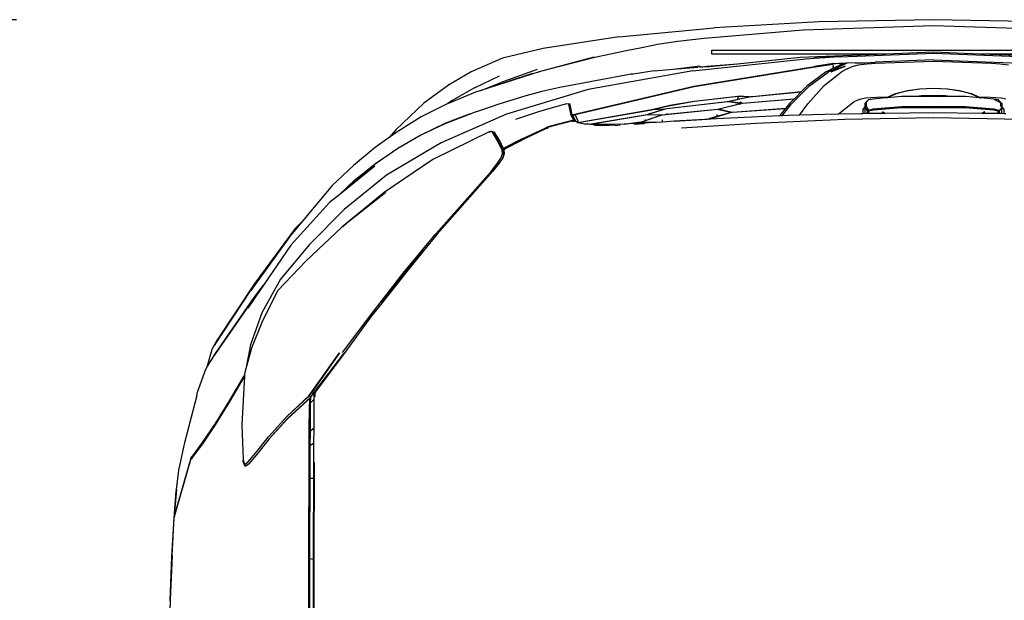
# Model space of a CAD drawing. Units: inches. Extents: x 0 to 4258, y 0 to 3769.
# Tile 13 of 30: x 3726 to 3763, y 3104 to 3126. Entities that reach past the tile are written whole.
import ezdxf

# ---------------------------------------------------------------- set-up
doc = ezdxf.new("R2010")
doc.units = ezdxf.units.IN
doc.header["$MEASUREMENT"] = 0
doc.layers.get('0').update_dxf_attribs({"color": 16})
doc.layers.add('A-ANNO-DIMS', color=250, linetype='Continuous', lineweight=18)
doc.layers.add('C-PKNG-VEHI', color=8, linetype='Continuous', lineweight=18)
doc.layers.add('Edges', color=250, linetype='Continuous')
doc.styles.get("Standard").update_dxf_attribs({"font": 'arial.ttf'})
doc.dimstyles.get("Standard").update_dxf_attribs({"dimtxt": 7, "dimasz": 0.18, "dimexe": 0.18, "dimexo": 0.0625, "dimgap": 0.09, "dimtad": 0, "dimtih": 1, "dimtoh": 1, "dimzin": 0, "dimdsep": 46, "dimlunit": 3, "dimtxsty": 'Standard', "dimcen": 0.09, "dimadec": 0, "dimazin": 0, "dimtfac": 1, "dimtofl": 0, "dimtmove": 0, "dimatfit": 3, "dimfxl": 1, "dimtolj": 1, "dimtzin": 0, "dimarcsym": 0})

# ---------------------------------------------------------------- blocks, each defined once
blk = doc.blocks.new('Nissan Qashqai pl')
at = {"layer": 'Edges'}
for p, q in [((7.3216, 11.6621), (7.3216, 12.1821)), ((7.3261, 12.1821), (7.3261, 11.9779)), ((7.3302, 12.0785), (7.3261, 11.9779)), ((7.298, 12.075), (7.2928, 11.9221)), ((7.2884, 12.0562), (7.2857, 11.9221)), ((7.3251, 11.9221), (7.3291, 12.0316)), ((7.3329, 11.9221), (7.3365, 12.0237)), ((7.4002, 11.9221), (7.4025, 12.026)), ((7.3373, 12.0004), (7.3386, 12.01)), ((7.3367, 11.99), (7.3373, 12.0004)), ((7.3768, 11.9954), (7.3775, 12.0015)), ((7.3775, 12.0015), (7.3786, 12.007)), ((7.3798, 11.9983), (7.3787, 11.9928)), ((7.3808, 11.9993), (7.3798, 11.9983)), ((7.3807, 11.9991), (7.3798, 11.9983)), ((7.38, 11.9953), (7.383, 12.0011)), ((7.3807, 11.9991), (7.3808, 11.9993)), ((7.381, 11.9993), (7.3807, 11.9991)), ((7.3808, 11.9993), (7.384, 12.0021)), ((7.381, 11.9993), (7.3808, 11.9993)), ((7.383, 12.0011), (7.381, 11.9993)), ((7.3866, 12.0011), (7.383, 12.0011)), ((7.384, 12.0021), (7.387, 12.0021)), ((7.3868, 12.002), (7.3866, 12.0011)), ((7.3875, 12.0011), (7.3866, 12.0011)), ((7.387, 12.0021), (7.3868, 12.002)), ((7.3909, 12.0051), (7.387, 12.0021)), ((7.387, 12.0021), (7.3885, 12.0021)), ((7.3885, 12.0021), (7.3925, 11.9993)), ((7.3955, 12.0021), (7.3885, 12.0021)), ((7.3904, 11.9928), (7.3916, 11.9983)), ((7.3956, 12.0051), (7.3909, 12.0051)), ((7.3929, 11.9981), (7.3917, 11.9926)), ((7.3925, 11.9993), (7.3958, 11.9993)), ((7.3925, 11.9993), (7.3929, 11.9981)), ((7.3958, 11.9981), (7.3929, 11.9981)), ((7.3955, 12.0021), (7.3958, 12.0018)), ((7.3959, 12.0049), (7.3956, 12.0051)), ((7.3959, 12.0051), (7.3956, 12.0051)), ((7.3958, 11.9981), (7.3956, 11.9801)), ((7.3959, 12.0049), (7.3958, 12.0018)), ((7.3958, 12.0018), (7.3958, 11.9993)), ((7.3958, 11.9993), (7.3958, 11.9981)), ((7.3959, 12.0071), (7.3959, 12.0051)), ((7.3959, 12.0051), (7.3959, 12.0049)), ((7.3343, 11.9221), (7.3367, 11.99)), ((7.3761, 11.9751), (7.3765, 11.989)), ((7.3765, 11.989), (7.3768, 11.9954)), ((7.3787, 11.9928), (7.3774, 11.9778)), ((7.3787, 11.9928), (7.38, 11.9953)), ((7.3876, 11.9595), (7.3904, 11.9928)), ((7.3917, 11.9926), (7.3889, 11.9594)), ((7.3261, 11.9764), (7.3238, 11.9221)), ((7.3261, 11.9764), (7.3261, 11.9779)), ((7.3724, 11.9667), (7.3761, 11.9751)), ((7.3771, 11.9757), (7.3727, 11.9658)), ((7.3773, 11.9759), (7.3759, 11.9595)), ((7.3761, 11.9751), (7.3769, 11.9767)), ((7.3769, 11.9767), (7.3771, 11.977)), ((7.3774, 11.9778), (7.3771, 11.9771)), ((7.3771, 11.9771), (7.3774, 11.9774)), ((7.3771, 11.9771), (7.3771, 11.977)), ((7.3773, 11.9759), (7.3771, 11.9757)), ((7.3774, 11.9774), (7.3773, 11.9759)), ((7.3774, 11.9774), (7.3774, 11.9778)), ((7.3938, 11.9823), (7.3956, 11.9801)), ((7.3956, 11.9788), (7.3938, 11.981)), ((7.3956, 11.9788), (7.3951, 11.9221)), ((7.3956, 11.9801), (7.3956, 11.9788)), ((7.369, 11.9536), (7.3724, 11.9667)), ((7.3727, 11.9658), (7.3693, 11.953)), ((7.3668, 11.9384), (7.369, 11.9536)), ((7.3693, 11.953), (7.3672, 11.9381)), ((7.3759, 11.9595), (7.3759, 11.9417)), ((7.3876, 11.8847), (7.3876, 11.9595)), ((7.3889, 11.9594), (7.3889, 11.8848)), ((7.3759, 11.9417), (7.3751, 11.9363)), ((7.3759, 11.9417), (7.3759, 11.9303)), ((7.3661, 11.9221), (7.3668, 11.9384)), ((7.3672, 11.9381), (7.3665, 11.9221)), ((7.3751, 11.9363), (7.3745, 11.9221)), ((7.3755, 11.9221), (7.3759, 11.9303)), ((7.3759, 11.9303), (7.3759, 11.9139)), ((7.2857, 11.9221), (7.2884, 11.7879)), ((7.2928, 11.9221), (7.298, 11.7692)), ((7.3238, 11.9221), (7.3261, 11.8662)), ((7.3291, 11.8126), (7.3251, 11.9221)), ((7.3329, 11.9221), (7.3354, 11.8539)), ((7.3367, 11.8541), (7.3343, 11.9221)), ((7.3668, 11.9057), (7.3661, 11.9221)), ((7.3665, 11.9221), (7.3672, 11.9061)), ((7.3745, 11.9221), (7.3751, 11.9078)), ((7.3759, 11.9139), (7.3755, 11.9221)), ((7.3951, 11.9221), (7.3956, 11.8653)), ((7.4025, 11.8181), (7.4002, 11.9221)), ((7.369, 11.8905), (7.3668, 11.9057)), ((7.3672, 11.9061), (7.3693, 11.8911)), ((7.3751, 11.9078), (7.3759, 11.9025)), ((7.3759, 11.9139), (7.3759, 11.9025)), ((7.3759, 11.9025), (7.3759, 11.8847)), ((7.3724, 11.8775), (7.369, 11.8905)), ((7.3693, 11.8911), (7.3727, 11.8783)), ((7.3759, 11.8847), (7.3773, 11.8682)), ((7.3904, 11.8513), (7.3876, 11.8847)), ((7.3889, 11.8848), (7.3917, 11.8516)), ((7.3761, 11.8691), (7.3724, 11.8775)), ((7.3727, 11.8783), (7.3771, 11.8685)), ((7.3261, 11.8662), (7.3302, 11.7656)), ((7.3261, 11.8662), (7.3261, 11.6621)), ((7.3765, 11.8551), (7.3761, 11.8691)), ((7.3769, 11.8674), (7.3761, 11.8691)), ((7.3771, 11.8671), (7.3769, 11.8674)), ((7.3771, 11.8685), (7.3773, 11.8682)), ((7.3771, 11.8671), (7.3771, 11.8671)), ((7.3771, 11.8671), (7.3774, 11.8664)), ((7.3774, 11.8668), (7.3771, 11.8671)), ((7.3773, 11.8682), (7.3774, 11.8668)), ((7.3774, 11.8668), (7.3774, 11.8664)), ((7.3774, 11.8664), (7.3787, 11.8513)), ((7.3938, 11.8632), (7.3956, 11.8653)), ((7.3956, 11.864), (7.3938, 11.8619)), ((7.3956, 11.8653), (7.3956, 11.864)), ((7.3956, 11.864), (7.3958, 11.8461)), ((7.3361, 11.8416), (7.3354, 11.8539)), ((7.3373, 11.8438), (7.3367, 11.8541)), ((7.3768, 11.8488), (7.3765, 11.8551)), ((7.3775, 11.8427), (7.3768, 11.8488)), ((7.3787, 11.8513), (7.3798, 11.8459)), ((7.3916, 11.8459), (7.3904, 11.8513)), ((7.3917, 11.8516), (7.3929, 11.8461)), ((7.3362, 11.8301), (7.3361, 11.8416)), ((7.3386, 11.8342), (7.3373, 11.8438)), ((7.3786, 11.8372), (7.3775, 11.8427)), ((7.3801, 11.8327), (7.3786, 11.8372)), ((7.3798, 11.8459), (7.3808, 11.8448)), ((7.3808, 11.8448), (7.3807, 11.8451)), ((7.3808, 11.8448), (7.381, 11.8448)), ((7.384, 11.8421), (7.3808, 11.8448)), ((7.383, 11.8431), (7.3875, 11.8431)), ((7.387, 11.8421), (7.384, 11.8421)), ((7.387, 11.8421), (7.3909, 11.8391)), ((7.3885, 11.8421), (7.387, 11.8421)), ((7.3875, 11.8431), (7.3916, 11.8459)), ((7.3925, 11.8448), (7.3885, 11.8421)), ((7.3955, 11.8421), (7.3885, 11.8421)), ((7.3909, 11.8391), (7.3956, 11.8391)), ((7.3929, 11.8461), (7.3925, 11.8448)), ((7.3958, 11.8448), (7.3925, 11.8448)), ((7.3929, 11.8461), (7.3958, 11.8461)), ((7.3958, 11.8423), (7.3955, 11.8421)), ((7.3956, 11.8391), (7.3959, 11.8392)), ((7.3956, 11.8391), (7.3959, 11.8391)), ((7.3958, 11.8461), (7.3958, 11.8448)), ((7.3958, 11.8448), (7.3958, 11.8423)), ((7.3958, 11.8423), (7.3959, 11.8392)), ((7.3959, 11.8392), (7.3959, 11.8391)), ((7.3959, 11.8391), (7.3959, 11.8371)), ((7.3959, 11.8371), (7.3966, 11.8103)), ((7.3362, 11.8301), (7.3365, 11.8204)), ((7.3407, 11.8266), (7.3386, 11.8342)), ((7.3432, 11.821), (7.3407, 11.8266)), ((7.3818, 11.8291), (7.3801, 11.8327)), ((7.3966, 11.8103), (7.3818, 11.8291)), ((7.3291, 11.8126), (7.3294, 11.8057)), ((7.3362, 11.8194), (7.3365, 11.8204)), ((7.3367, 11.8196), (7.3362, 11.8194)), ((7.3365, 11.812), (7.3362, 11.8194)), ((7.3365, 11.8204), (7.3471, 11.7987)), ((7.3369, 11.8155), (7.3374, 11.8165)), ((7.3369, 11.8113), (7.3369, 11.8155)), ((7.3369, 11.8155), (7.338, 11.8151)), ((7.3374, 11.8165), (7.338, 11.8151)), ((7.338, 11.8151), (7.343, 11.8045)), ((7.3401, 11.8186), (7.3431, 11.8112)), ((7.347, 11.8021), (7.3401, 11.8186)), ((7.3432, 11.821), (7.3468, 11.8142)), ((7.363, 11.794), (7.3468, 11.8142)), ((7.4072, 11.7142), (7.4025, 11.8181)), ((7.3301, 11.7949), (7.3294, 11.8057)), ((7.3295, 11.8012), (7.3309, 11.7822)), ((7.3295, 11.8012), (7.3301, 11.7949)), ((7.3369, 11.8047), (7.3365, 11.812)), ((7.3369, 11.8113), (7.3377, 11.8044)), ((7.3369, 11.8047), (7.3405, 11.7825)), ((7.3377, 11.8042), (7.3377, 11.8044)), ((7.341, 11.7837), (7.3377, 11.8042)), ((7.343, 11.8045), (7.3396, 11.8043)), ((7.3396, 11.8043), (7.3431, 11.8042)), ((7.343, 11.8045), (7.3431, 11.8042)), ((7.3431, 11.8112), (7.347, 11.8021)), ((7.3431, 11.8042), (7.3469, 11.7961)), ((7.3966, 11.8103), (7.3978, 11.7651)), ((7.3309, 11.7822), (7.3301, 11.7949)), ((7.3469, 11.7961), (7.3631, 11.774)), ((7.3633, 11.7767), (7.3471, 11.7987)), ((7.3842, 11.7749), (7.363, 11.794)), ((7.2884, 11.7879), (7.2951, 11.6651)), ((7.3317, 11.7724), (7.3309, 11.7822)), ((7.3635, 11.6409), (7.3405, 11.7825)), ((7.3426, 11.7735), (7.341, 11.7837)), ((7.298, 11.7692), (7.3078, 11.6532)), ((7.3455, 11.64), (7.3317, 11.7724)), ((7.364, 11.6413), (7.3426, 11.7735)), ((7.3631, 11.774), (7.3701, 11.7671)), ((7.3845, 11.7558), (7.3633, 11.7767)), ((7.3759, 11.7101), (7.3701, 11.7671)), ((7.3701, 11.7671), (7.3704, 11.7668)), ((7.3704, 11.7668), (7.3761, 11.71)), ((7.3704, 11.7668), (7.3783, 11.759)), ((7.3978, 11.7651), (7.3842, 11.7749)), ((7.3302, 11.7656), (7.3378, 11.6921)), ((7.3836, 11.6983), (7.3783, 11.759)), ((7.3783, 11.759), (7.3788, 11.7585)), ((7.3788, 11.7585), (7.384, 11.6982)), ((7.3788, 11.7585), (7.3841, 11.7532)), ((7.3985, 11.7448), (7.3845, 11.7558)), ((7.3978, 11.7651), (7.3982, 11.7521)), ((7.3841, 11.7532), (7.3896, 11.7488)), ((7.3941, 11.6865), (7.3896, 11.7488)), ((7.3896, 11.7488), (7.3903, 11.7483)), ((7.3903, 11.7483), (7.3945, 11.6865)), ((7.3903, 11.7483), (7.3986, 11.7417)), ((7.3982, 11.7521), (7.3985, 11.7448)), ((7.3985, 11.7448), (7.3986, 11.7417)), ((7.3986, 11.7417), (7.4018, 11.6678)), ((7.376, 11.7081), (7.3759, 11.7101)), ((7.3761, 11.71), (7.3763, 11.7081)), ((7.4124, 11.6265), (7.4072, 11.7142)), ((7.375, 11.6957), (7.376, 11.7081)), ((7.3762, 11.7062), (7.3757, 11.6959)), ((7.3762, 11.7062), (7.3764, 11.7061)), ((7.3763, 11.7081), (7.3813, 11.6842)), ((7.3764, 11.7061), (7.3792, 11.6924)), ((7.3824, 11.6955), (7.3836, 11.6983)), ((7.3835, 11.6973), (7.3824, 11.6955)), ((7.3835, 11.6973), (7.3836, 11.6983)), ((7.3836, 11.6975), (7.3835, 11.6973)), ((7.3836, 11.6975), (7.3836, 11.6983)), ((7.384, 11.6982), (7.3836, 11.6975)), ((7.3378, 11.6921), (7.3407, 11.6563)), ((7.3378, 11.6921), (7.34, 11.671)), ((7.3813, 11.642), (7.375, 11.6957)), ((7.3757, 11.6959), (7.3756, 11.6933)), ((7.3792, 11.6924), (7.3756, 11.6933)), ((7.3756, 11.6933), (7.3815, 11.6413)), ((7.3757, 11.6959), (7.3757, 11.6959)), ((7.3812, 11.6823), (7.3792, 11.6924)), ((7.3817, 11.6844), (7.3832, 11.6949)), ((7.3838, 11.6944), (7.382, 11.6823)), ((7.3834, 11.6959), (7.3824, 11.6955)), ((7.3824, 11.6955), (7.3832, 11.6949)), ((7.3832, 11.695), (7.3824, 11.6955)), ((7.3832, 11.695), (7.3834, 11.6959)), ((7.3838, 11.6947), (7.3832, 11.695)), ((7.3832, 11.6949), (7.3838, 11.6944)), ((7.3837, 11.696), (7.3834, 11.6959)), ((7.3844, 11.6963), (7.3837, 11.696)), ((7.3838, 11.6947), (7.3837, 11.696)), ((7.3843, 11.6944), (7.3838, 11.6947)), ((7.3843, 11.6942), (7.3838, 11.6944)), ((7.3843, 11.6944), (7.3844, 11.6963)), ((7.3843, 11.6942), (7.3843, 11.6944)), ((7.3877, 11.6803), (7.3843, 11.6942)), ((7.3844, 11.6963), (7.3903, 11.6725)), ((7.3939, 11.6846), (7.3941, 11.6865)), ((7.3945, 11.6865), (7.3951, 11.6835)), ((7.3815, 11.6804), (7.3812, 11.6823)), ((7.3813, 11.6842), (7.3817, 11.6844)), ((7.3817, 11.6841), (7.3813, 11.6842)), ((7.3899, 11.6094), (7.3815, 11.6804)), ((7.3817, 11.6841), (7.3817, 11.6844)), ((7.382, 11.6823), (7.382, 11.6803)), ((7.382, 11.6803), (7.3903, 11.6095)), ((7.3874, 11.6803), (7.3877, 11.6803)), ((7.3901, 11.6707), (7.3877, 11.6803)), ((7.3909, 11.6728), (7.3939, 11.6846)), ((7.3943, 11.6827), (7.3913, 11.6705)), ((7.3943, 11.6827), (7.3949, 11.6826)), ((7.3943, 11.6827), (7.395, 11.6825)), ((7.395, 11.6825), (7.3949, 11.6826)), ((7.399, 11.6686), (7.395, 11.6825)), ((7.3951, 11.6835), (7.4021, 11.6609)), ((7.3059, 11.5532), (7.2951, 11.6651)), ((7.3261, 11.6621), (7.3216, 11.6621)), ((7.34, 11.671), (7.341, 11.6594)), ((7.3905, 11.6687), (7.3901, 11.6707)), ((7.3909, 11.6728), (7.3903, 11.6725)), ((7.3909, 11.6725), (7.3903, 11.6725)), ((7.3966, 11.6095), (7.3905, 11.6687)), ((7.3909, 11.6725), (7.3909, 11.6728)), ((7.3913, 11.6705), (7.3911, 11.6687)), ((7.3911, 11.6687), (7.3977, 11.6042)), ((7.399, 11.6686), (7.3967, 11.6686)), ((7.4017, 11.6592), (7.399, 11.6686)), ((7.4018, 11.6678), (7.4022, 11.6609)), ((7.3078, 11.6532), (7.3113, 11.6224)), ((7.3407, 11.6563), (7.3413, 11.6509)), ((7.341, 11.6594), (7.3413, 11.6511)), ((7.341, 11.648), (7.3413, 11.6509)), ((7.3413, 11.6511), (7.3413, 11.6509)), ((7.3413, 11.6509), (7.3415, 11.6488)), ((7.4022, 11.6571), (7.4017, 11.6592)), ((7.4022, 11.6609), (7.4021, 11.6609)), ((7.4022, 11.6609), (7.4021, 11.6609)), ((7.4022, 11.6609), (7.4048, 11.618)), ((7.4022, 11.6609), (7.4022, 11.6609)), ((7.4048, 11.618), (7.4022, 11.6571)), ((7.3401, 11.648), (7.34, 11.648)), ((7.3438, 11.6167), (7.34, 11.648)), ((7.341, 11.648), (7.3401, 11.648)), ((7.3414, 11.648), (7.341, 11.648)), ((7.341, 11.648), (7.3414, 11.648)), ((7.3438, 11.6167), (7.3412, 11.646)), ((7.3455, 11.64), (7.3676, 11.5172)), ((7.3971, 11.4981), (7.3635, 11.6409)), ((7.3968, 11.5018), (7.364, 11.6413)), ((7.3869, 11.6094), (7.3813, 11.642)), ((7.3815, 11.6413), (7.3864, 11.6131)), ((7.3113, 11.6224), (7.3149, 11.5984)), ((7.3457, 11.5947), (7.3438, 11.6167)), ((7.4048, 11.618), (7.4057, 11.6042)), ((7.3864, 11.6131), (7.3909, 11.5933)), ((7.3912, 11.5914), (7.3869, 11.6094)), ((7.3901, 11.6073), (7.3899, 11.6094)), ((7.391, 11.5935), (7.3901, 11.6073)), ((7.3903, 11.6095), (7.3908, 11.6076)), ((7.3906, 11.6055), (7.391, 11.6055)), ((7.3906, 11.6055), (7.391, 11.6054)), ((7.3906, 11.6055), (7.3914, 11.5914)), ((7.3908, 11.6076), (7.3965, 11.5881)), ((7.391, 11.6054), (7.391, 11.6055)), ((7.3967, 11.5862), (7.391, 11.6054)), ((7.3966, 11.6095), (7.3957, 11.6095)), ((7.3972, 11.6042), (7.3966, 11.6095)), ((7.3149, 11.5984), (7.3186, 11.58)), ((7.3457, 11.5947), (7.3494, 11.57)), ((7.391, 11.5935), (7.3909, 11.5933)), ((7.391, 11.5934), (7.3909, 11.5933)), ((7.3968, 11.5882), (7.3972, 11.6021)), ((7.3972, 11.6021), (7.3972, 11.6042)), ((7.3977, 11.6003), (7.3973, 11.5862)), ((7.3977, 11.6042), (7.3982, 11.6022)), ((7.3977, 11.6003), (7.3983, 11.6002)), ((7.3977, 11.6003), (7.3983, 11.6001)), ((7.3982, 11.6022), (7.4048, 11.5829)), ((7.3983, 11.6001), (7.3983, 11.6002)), ((7.4038, 11.5843), (7.3983, 11.6001)), ((7.4057, 11.6042), (7.4032, 11.6042)), ((7.4053, 11.5831), (7.4061, 11.5969)), ((7.4057, 11.6042), (7.4061, 11.597)), ((7.4061, 11.5969), (7.4061, 11.597)), ((7.4061, 11.5969), (7.4064, 11.5919)), ((7.3916, 11.5894), (7.3912, 11.5914)), ((7.3914, 11.5914), (7.3917, 11.5895)), ((7.4062, 11.5053), (7.3916, 11.5894)), ((7.3917, 11.5895), (7.4065, 11.505)), ((7.3968, 11.5882), (7.3965, 11.5881)), ((7.3971, 11.5842), (7.3967, 11.5862)), ((7.3968, 11.5882), (7.3973, 11.5884)), ((7.4083, 11.5184), (7.3971, 11.5842)), ((7.3973, 11.5862), (7.3975, 11.5843)), ((7.3975, 11.5843), (7.4084, 11.5198)), ((7.4038, 11.5843), (7.4028, 11.5843)), ((7.4049, 11.5811), (7.4038, 11.5843)), ((7.4053, 11.5831), (7.4048, 11.5829)), ((7.4053, 11.583), (7.4048, 11.5829)), ((7.406, 11.5834), (7.4053, 11.5831)), ((7.406, 11.5833), (7.4053, 11.583)), ((7.4053, 11.583), (7.4053, 11.5831)), ((7.406, 11.5833), (7.4058, 11.581)), ((7.4064, 11.5919), (7.406, 11.5834)), ((7.406, 11.5834), (7.406, 11.5833)), ((7.4064, 11.5919), (7.4069, 11.5844)), ((7.4069, 11.5844), (7.4079, 11.5644)), ((7.4081, 11.5711), (7.4075, 11.5828)), ((7.3186, 11.58), (7.3223, 11.5616)), ((7.3494, 11.57), (7.3497, 11.5674)), ((7.3494, 11.57), (7.3498, 11.5674)), ((7.4054, 11.5791), (7.4049, 11.5811)), ((7.4081, 11.5593), (7.4054, 11.5791)), ((7.4058, 11.581), (7.4059, 11.579)), ((7.4059, 11.579), (7.4079, 11.5644)), ((7.3223, 11.5616), (7.3261, 11.5433)), ((7.3497, 11.5674), (7.3653, 11.4838)), ((7.4079, 11.5644), (7.4081, 11.5604)), ((7.4079, 11.5644), (7.4081, 11.5629)), ((7.4081, 11.5604), (7.4081, 11.5593)), ((7.4081, 11.5593), (7.4087, 11.5405)), ((7.3059, 11.5532), (7.3193, 11.4645)), ((7.4092, 11.5416), (7.409, 11.5485)), ((7.4096, 11.549), (7.4092, 11.5521)), ((7.4093, 11.5546), (7.4095, 11.5529)), ((7.3261, 11.5433), (7.33, 11.5249)), ((7.4087, 11.5405), (7.4087, 11.5246)), ((7.4092, 11.5258), (7.4092, 11.5416)), ((7.3297, 11.5237), (7.3467, 11.4596)), ((7.33, 11.5249), (7.3467, 11.4596)), ((7.4087, 11.5246), (7.4084, 11.5198)), ((7.4091, 11.5235), (7.4092, 11.5258)), ((7.3676, 11.5172), (7.3963, 11.4215)), ((7.408, 11.5129), (7.4066, 11.5052)), ((7.4083, 11.5184), (7.408, 11.5129)), ((7.4084, 11.5198), (7.4083, 11.5184)), ((7.4046, 11.5053), (7.3968, 11.5018)), ((7.398, 11.4993), (7.3968, 11.5018)), ((7.398, 11.4993), (7.4048, 11.5024)), ((7.4012, 11.5001), (7.4033, 11.5014)), ((7.403, 11.5005), (7.4026, 11.5002)), ((7.403, 11.5005), (7.4028, 11.5004)), ((7.4033, 11.5007), (7.403, 11.5005)), ((7.4033, 11.5014), (7.4042, 11.502)), ((7.4042, 11.502), (7.4033, 11.5007)), ((7.4033, 11.5005), (7.4033, 11.5007)), ((7.4034, 11.5005), (7.4033, 11.5005)), ((7.4101, 11.4733), (7.4033, 11.5005)), ((7.4043, 11.5016), (7.404, 11.5012)), ((7.4043, 11.5014), (7.404, 11.5012)), ((7.404, 11.5012), (7.4108, 11.4738)), ((7.4042, 11.502), (7.4044, 11.502)), ((7.4043, 11.5016), (7.4042, 11.502)), ((7.4044, 11.502), (7.4043, 11.5016)), ((7.4046, 11.5016), (7.4043, 11.5014)), ((7.4043, 11.5014), (7.4043, 11.5016)), ((7.4045, 11.5008), (7.4043, 11.5014)), ((7.4046, 11.5023), (7.4044, 11.502)), ((7.4044, 11.502), (7.4046, 11.502)), ((7.4048, 11.5008), (7.4045, 11.5008)), ((7.405, 11.4985), (7.4045, 11.5008)), ((7.4062, 11.5053), (7.4046, 11.5053)), ((7.4046, 11.5023), (7.4048, 11.5024)), ((7.405, 11.5023), (7.4046, 11.5023)), ((7.4046, 11.5023), (7.4046, 11.502)), ((7.4046, 11.502), (7.4047, 11.5018)), ((7.4046, 11.502), (7.4048, 11.502)), ((7.4047, 11.5018), (7.4046, 11.5016)), ((7.4048, 11.502), (7.4047, 11.5018)), ((7.4048, 11.5024), (7.4052, 11.5027)), ((7.4052, 11.5026), (7.4048, 11.5024)), ((7.405, 11.5023), (7.4048, 11.502)), ((7.4052, 11.5026), (7.405, 11.5023)), ((7.4063, 11.5047), (7.4052, 11.5027)), ((7.4052, 11.5027), (7.4052, 11.5026)), ((7.4063, 11.5047), (7.4062, 11.5053)), ((7.4065, 11.505), (7.4063, 11.5047)), ((7.4066, 11.5052), (7.4065, 11.505)), ((7.3853, 11.4958), (7.3841, 11.4956)), ((7.3844, 11.4916), (7.3841, 11.4956)), ((7.3846, 11.4946), (7.3844, 11.4916)), ((7.3844, 11.4916), (7.3914, 11.4667)), ((7.3976, 11.4971), (7.3846, 11.4946)), ((7.3853, 11.4958), (7.3846, 11.4946)), ((7.3853, 11.4958), (7.3971, 11.4981)), ((7.3971, 11.4981), (7.3983, 11.4983)), ((7.4026, 11.5002), (7.3976, 11.4971)), ((7.4012, 11.5001), (7.398, 11.4993)), ((7.3983, 11.4983), (7.4012, 11.5001)), ((7.3653, 11.4838), (7.3699, 11.4629)), ((7.3914, 11.4667), (7.3925, 11.4629)), ((7.4115, 11.4695), (7.4101, 11.4733)), ((7.4108, 11.4738), (7.4122, 11.47)), ((7.4131, 11.4659), (7.4115, 11.4695)), ((7.4122, 11.47), (7.4139, 11.4664)), ((7.4126, 11.47), (7.4125, 11.4702)), ((7.4132, 11.4685), (7.4126, 11.47)), ((7.4255, 11.4398), (7.4131, 11.4659)), ((7.4139, 11.4664), (7.4267, 11.4401)), ((7.3193, 11.4645), (7.3309, 11.4166)), ((7.344, 11.4572), (7.3596, 11.4139)), ((7.3489, 11.4517), (7.3467, 11.4596)), ((7.3467, 11.4596), (7.3686, 11.3913)), ((7.3699, 11.4629), (7.375, 11.4442)), ((7.3925, 11.4629), (7.3937, 11.4591)), ((7.3937, 11.4591), (7.4029, 11.4321)), ((7.3489, 11.4517), (7.3686, 11.3913)), ((7.375, 11.4442), (7.3799, 11.4278)), ((7.4255, 11.4398), (7.4367, 11.4174)), ((7.4379, 11.4179), (7.4267, 11.4401)), ((7.3799, 11.4278), (7.3845, 11.4136)), ((7.3963, 11.4215), (7.4302, 11.3449)), ((7.4375, 11.42), (7.4384, 11.4182)), ((7.3309, 11.4166), (7.347, 11.3798)), ((7.3655, 11.3837), (7.3514, 11.4133)), ((7.3686, 11.3913), (7.3596, 11.4139)), ((7.3845, 11.4136), (7.3925, 11.3899)), ((7.4282, 11.4113), (7.4169, 11.4044)), ((7.417, 11.4065), (7.4283, 11.4135)), ((7.4296, 11.4129), (7.4183, 11.406)), ((7.4387, 11.4162), (7.4282, 11.4113)), ((7.4283, 11.4135), (7.4359, 11.417)), ((7.4296, 11.4129), (7.4383, 11.417)), ((7.4359, 11.417), (7.4367, 11.4174)), ((7.4383, 11.417), (7.4367, 11.4174)), ((7.4379, 11.4179), (7.4384, 11.4182)), ((7.4389, 11.4173), (7.4379, 11.4179)), ((7.4383, 11.417), (7.4379, 11.4179)), ((7.4389, 11.4173), (7.4383, 11.417)), ((7.4384, 11.4182), (7.4387, 11.4183)), ((7.4387, 11.4183), (7.443, 11.4188)), ((7.4431, 11.4166), (7.4387, 11.4162)), ((7.4389, 11.4173), (7.44, 11.4178)), ((7.4442, 11.4183), (7.44, 11.4178)), ((7.443, 11.4188), (7.4477, 11.4172)), ((7.4479, 11.4149), (7.4431, 11.4166)), ((7.4477, 11.4172), (7.4442, 11.4183)), ((7.4477, 11.4172), (7.4541, 11.4128)), ((7.4541, 11.4108), (7.4479, 11.4149)), ((7.4541, 11.4128), (7.4638, 11.4051)), ((7.4635, 11.4034), (7.4541, 11.4108)), ((7.4167, 11.4049), (7.417, 11.4065)), ((7.4172, 11.4047), (7.4167, 11.4049)), ((7.4169, 11.4036), (7.4167, 11.4049)), ((7.4172, 11.4047), (7.4169, 11.4044)), ((7.4169, 11.4044), (7.4169, 11.4036)), ((7.4172, 11.4018), (7.4169, 11.4036)), ((7.4169, 11.4036), (7.4169, 11.403)), ((7.4169, 11.403), (7.4172, 11.4011)), ((7.4183, 11.406), (7.4172, 11.4047)), ((7.4174, 11.4013), (7.4172, 11.4018)), ((7.4172, 11.4011), (7.4498, 11.3349)), ((7.4174, 11.4013), (7.4175, 11.4012)), ((7.5369, 11.3385), (7.4635, 11.4034)), ((7.4638, 11.4051), (7.5371, 11.34)), ((7.3686, 11.3913), (7.3707, 11.3849)), ((7.3925, 11.3899), (7.3938, 11.3859)), ((7.3938, 11.3859), (7.3951, 11.3822)), ((7.347, 11.3798), (7.3624, 11.3535)), ((7.3655, 11.3837), (7.3805, 11.3576)), ((7.3707, 11.3849), (7.3843, 11.3522)), ((7.3951, 11.3822), (7.3965, 11.3787)), ((7.3962, 11.3781), (7.3965, 11.3787)), ((7.4071, 11.3493), (7.3962, 11.3781)), ((7.3965, 11.3787), (7.3969, 11.3777)), ((7.3969, 11.3777), (7.4078, 11.349)), ((7.3624, 11.3535), (7.3837, 11.3245)), ((7.3805, 11.3576), (7.3843, 11.3522)), ((7.3843, 11.3522), (7.3845, 11.3517)), ((7.3845, 11.3517), (7.3997, 11.3215)), ((7.4205, 11.3212), (7.4071, 11.3493)), ((7.4078, 11.349), (7.4211, 11.321)), ((7.4302, 11.3449), (7.4679, 11.2807)), ((7.5371, 11.34), (7.5568, 11.324)), ((7.4498, 11.3349), (7.4884, 11.2778)), ((7.5827, 11.3001), (7.5369, 11.3385)), ((7.3837, 11.3245), (7.4147, 11.2918)), ((7.3997, 11.3215), (7.4166, 11.2939)), ((7.4363, 11.294), (7.4205, 11.3212)), ((7.4211, 11.321), (7.4369, 11.2938)), ((7.584, 11.3013), (7.5568, 11.324)), ((7.5568, 11.324), (7.5829, 11.303)), ((7.4166, 11.2939), (7.4239, 11.2837)), ((7.4542, 11.2677), (7.4363, 11.294)), ((7.4369, 11.2938), (7.4549, 11.2675)), ((7.6296, 11.2639), (7.5827, 11.3001)), ((7.5829, 11.303), (7.618, 11.275)), ((7.618, 11.275), (7.584, 11.3013)), ((7.4147, 11.2918), (7.4239, 11.2837)), ((7.4239, 11.2837), (7.4354, 11.2675)), ((7.4679, 11.2807), (7.5081, 11.2311)), ((7.4882, 11.2797), (7.5243, 11.2341)), ((7.4884, 11.2778), (7.5289, 11.2283)), ((7.618, 11.275), (7.6301, 11.2654)), ((7.4354, 11.2675), (7.4565, 11.2419)), ((7.4744, 11.2427), (7.4542, 11.2677)), ((7.4549, 11.2675), (7.475, 11.2426)), ((7.4574, 11.267), (7.4885, 11.2283)), ((7.676, 11.2289), (7.6296, 11.2639)), ((7.6301, 11.2654), (7.6306, 11.2651)), ((7.6306, 11.2651), (7.6306, 11.265)), ((7.6306, 11.265), (7.6373, 11.2601)), ((7.6373, 11.2601), (7.6769, 11.2312)), ((7.4565, 11.2419), (7.4801, 11.2168)), ((7.4918, 11.2242), (7.4744, 11.2427)), ((7.475, 11.2426), (7.477, 11.2404)), ((7.477, 11.2404), (7.4765, 11.2411)), ((7.477, 11.2405), (7.4775, 11.2399)), ((7.4784, 11.2388), (7.477, 11.2404)), ((7.477, 11.2404), (7.4775, 11.2399)), ((7.4775, 11.2399), (7.4787, 11.2385)), ((7.4775, 11.2399), (7.4787, 11.2387)), ((7.4787, 11.2387), (7.4782, 11.2392)), ((7.4795, 11.2377), (7.4787, 11.2387)), ((7.4787, 11.2387), (7.4885, 11.2283)), ((7.4885, 11.2283), (7.4918, 11.2242)), ((7.4918, 11.2242), (7.5001, 11.2139)), ((7.5081, 11.2311), (7.5492, 11.1902)), ((7.5243, 11.2341), (7.5286, 11.2296)), ((7.5289, 11.2283), (7.5687, 11.1862)), ((7.7261, 11.1898), (7.6762, 11.2256)), ((7.6762, 11.2256), (7.7233, 11.1928)), ((7.6769, 11.2312), (7.7194, 11.1992)), ((7.7232, 11.1955), (7.6771, 11.2307)), ((7.4801, 11.2168), (7.5217, 11.1823)), ((7.5001, 11.2139), (7.5501, 11.1684)), ((7.5492, 11.1902), (7.59, 11.1565)), ((7.7194, 11.1992), (7.7232, 11.1966)), ((7.7232, 11.1966), (7.7279, 11.1965)), ((7.7281, 11.1918), (7.7232, 11.1955)), ((7.7232, 11.1955), (7.7245, 11.1955)), ((7.7267, 11.1902), (7.7233, 11.1928)), ((7.7247, 11.1954), (7.7245, 11.1955)), ((7.7245, 11.1955), (7.7294, 11.1955)), ((7.7261, 11.1898), (7.7507, 11.1638)), ((7.7286, 11.1881), (7.7267, 11.1902)), ((7.7281, 11.1918), (7.7299, 11.1904)), ((7.7349, 11.1917), (7.7281, 11.1918)), ((7.753, 11.1648), (7.7281, 11.1918)), ((7.7294, 11.1955), (7.731, 11.1955)), ((7.7299, 11.1904), (7.7324, 11.1876)), ((7.7299, 11.1904), (7.7364, 11.1904)), ((7.731, 11.1955), (7.7349, 11.1917)), ((7.731, 11.1955), (7.764, 11.1953)), ((7.768, 11.1915), (7.7349, 11.1917)), ((7.7363, 11.1904), (7.7364, 11.1904)), ((7.7694, 11.1901), (7.7364, 11.1904)), ((7.764, 11.1953), (7.7636, 11.1957)), ((7.768, 11.1915), (7.764, 11.1953)), ((7.764, 11.1953), (7.7662, 11.1953)), ((7.7659, 11.1957), (7.7662, 11.1953)), ((7.7662, 11.1953), (7.7668, 11.1946)), ((7.7662, 11.1953), (7.7811, 11.1952)), ((7.7692, 11.1915), (7.768, 11.1915)), ((7.7694, 11.1901), (7.7687, 11.1908)), ((7.7844, 11.1913), (7.7692, 11.1915)), ((7.7707, 11.1901), (7.7694, 11.1901)), ((7.7851, 11.19), (7.7707, 11.1901)), ((7.7811, 11.1952), (7.7809, 11.1958)), ((7.7814, 11.1946), (7.7811, 11.1952)), ((7.7811, 11.1952), (7.7822, 11.1952)), ((7.7822, 11.1952), (7.7819, 11.1958)), ((7.7822, 11.1952), (7.8057, 11.195)), ((7.7844, 11.1913), (7.7822, 11.1952)), ((7.8078, 11.1911), (7.7844, 11.1913)), ((7.7846, 11.1909), (7.7851, 11.19)), ((7.8083, 11.1898), (7.7851, 11.19)), ((7.8048, 11.1959), (7.8233, 11.1958)), ((7.8057, 11.195), (7.8233, 11.195)), ((7.8233, 11.1911), (7.8078, 11.1911)), ((7.904, 11.1894), (7.8083, 11.1898)), ((7.8233, 11.195), (7.8233, 11.1958)), ((7.8233, 11.1958), (7.9014, 11.1955)), ((7.8233, 11.195), (7.902, 11.1947)), ((7.8233, 11.1911), (7.8233, 11.195)), ((7.8233, 11.1899), (7.8233, 11.1911)), ((7.9036, 11.1907), (7.8233, 11.1911)), ((7.9014, 11.1955), (7.9185, 11.1955)), ((7.902, 11.1947), (7.9183, 11.1947)), ((7.9176, 11.1908), (7.9036, 11.1907)), ((8.0276, 11.1896), (7.904, 11.1894)), ((7.9183, 11.1947), (7.9176, 11.1908)), ((8.0275, 11.1909), (7.9176, 11.1908)), ((7.9185, 11.1955), (7.9183, 11.1947)), ((7.9183, 11.1947), (8.0275, 11.1948)), ((7.9185, 11.1955), (8.0273, 11.1957)), ((7.5304, 11.1737), (7.5217, 11.1823)), ((7.5217, 11.1823), (7.5387, 11.1682)), ((7.5687, 11.1862), (7.6032, 11.1533)), ((7.7507, 11.1638), (7.7286, 11.1881)), ((7.7324, 11.1876), (7.7539, 11.1642)), ((7.5304, 11.1737), (7.5946, 11.1262)), ((7.5387, 11.1682), (7.6031, 11.1217)), ((7.5501, 11.1684), (7.5969, 11.1365)), ((7.59, 11.1565), (7.6295, 11.1344)), ((7.7748, 11.1423), (7.7507, 11.1638)), ((7.753, 11.1648), (7.7772, 11.1431)), ((7.7539, 11.1642), (7.7772, 11.1431)), ((7.6032, 11.1533), (7.6386, 11.1353)), ((7.7772, 11.1431), (7.7959, 11.1281)), ((7.6113, 11.1256), (7.5969, 11.1365)), ((7.5969, 11.1365), (7.6021, 11.1329)), ((7.6021, 11.1329), (7.6118, 11.1255)), ((7.6021, 11.1329), (7.6237, 11.1181)), ((7.6295, 11.1344), (7.667, 11.1212)), ((7.6386, 11.1353), (7.6708, 11.1225)), ((7.7938, 11.1271), (7.7748, 11.1423)), ((7.5946, 11.1262), (7.6608, 11.0825)), ((7.6676, 11.0791), (7.6024, 11.1221)), ((7.6759, 11.0809), (7.6113, 11.1256)), ((7.6118, 11.1255), (7.6799, 11.0783)), ((7.667, 11.1212), (7.6949, 11.1158)), ((7.6708, 11.1225), (7.6949, 11.1158)), ((7.8045, 11.1179), (7.7938, 11.1271)), ((7.7959, 11.1281), (7.8062, 11.1192)), ((7.6949, 11.1158), (7.701, 11.1141)), ((7.701, 11.1141), (7.7024, 11.1141)), ((7.7038, 11.1132), (7.7024, 11.1141)), ((7.7024, 11.1141), (7.7034, 11.114)), ((7.7034, 11.114), (7.7056, 11.1128)), ((7.7034, 11.114), (7.7608, 11.1112)), ((7.7325, 11.0966), (7.7038, 11.1132)), ((7.7056, 11.1128), (7.7341, 11.0963)), ((7.7608, 11.1112), (7.8014, 11.1124)), ((7.8014, 11.1124), (7.8022, 11.1126)), ((7.8022, 11.1126), (7.8072, 11.1141)), ((7.8037, 11.1126), (7.8022, 11.1126)), ((7.8096, 11.1148), (7.8037, 11.1126)), ((7.8072, 11.1141), (7.8045, 11.1179)), ((7.8087, 11.1159), (7.8062, 11.1192)), ((7.8062, 11.1192), (7.8066, 11.1188)), ((7.8066, 11.1188), (7.8096, 11.1148)), ((7.8072, 11.1141), (7.8087, 11.1159)), ((7.7591, 11.08), (7.7325, 11.0966)), ((7.7341, 11.0963), (7.7606, 11.0798)), ((7.6712, 11.0767), (7.6608, 11.0825)), ((7.6721, 11.0762), (7.6712, 11.0767)), ((7.6926, 11.0705), (7.6721, 11.0762)), ((7.6793, 11.0784), (7.6759, 11.0809)), ((7.6802, 11.0782), (7.6793, 11.0784)), ((7.6802, 11.0782), (7.6799, 11.0783)), ((7.6809, 11.0777), (7.6802, 11.0782)), ((7.6926, 11.0705), (7.6809, 11.0777)), ((7.7814, 11.065), (7.7591, 11.08)), ((7.7606, 11.0798), (7.7828, 11.0649)), ((7.6953, 11.0688), (7.6926, 11.0705)), ((7.7223, 11.059), (7.6953, 11.0688)), ((7.797, 11.0534), (7.7814, 11.065)), ((7.7828, 11.0649), (7.7984, 11.0533)), ((7.7262, 11.0581), (7.7223, 11.059)), ((7.7262, 11.0581), (7.7819, 11.0438)), ((7.797, 11.0534), (7.797, 11.0534)), ((7.7998, 11.0513), (7.797, 11.0534)), ((7.7984, 11.0533), (7.8007, 11.0516)), ((7.7998, 11.0513), (7.8676, 11.0318)), ((7.8007, 11.0516), (7.8002, 11.0517)), ((7.8007, 11.0516), (7.8012, 11.0513)), ((7.8681, 11.032), (7.8012, 11.0513)), ((7.7819, 11.0438), (7.7848, 11.043)), ((7.7848, 11.043), (7.8087, 11.038)), ((7.8087, 11.038), (7.8106, 11.0377)), ((7.8107, 11.0377), (7.8106, 11.0377)), ((7.8363, 11.0344), (7.8107, 11.0377)), ((7.8381, 11.0342), (7.8363, 11.0344)), ((7.8363, 11.0344), (7.8676, 11.0318)), ((7.87, 11.0315), (7.8381, 11.0342)), ((7.8681, 11.032), (7.8676, 11.0318)), ((7.8681, 11.032), (7.869, 11.0317)), ((7.9137, 11.0292), (7.869, 11.0317)), ((7.9151, 11.029), (7.87, 11.0315)), ((7.9137, 11.0292), (7.9658, 11.027)), ((7.9668, 11.0268), (7.9151, 11.029)), ((7.9658, 11.027), (8.016, 11.0253))]:
    blk.add_line(p, q, dxfattribs=at)
blk = doc.blocks.new('car')
blk.add_blockref('Nissan Qashqai pl', (-9.7433, -11.9151))
blk = doc.blocks.new('*D66')
at = {"layer": 'A-ANNO-DIMS', "color": 0, "lineweight": -2, "transparency": 16777216}
for p, q in [((3725.517, 3125.846), (3703.936, 3125.846)), ((3704.116, 3125.666), (3704.116, 3058.01)), ((3704.116, 2982.935), (3704.116, 3050.591)), ((3725.517, 2982.755), (3703.936, 2982.755))]:
    blk.add_line(p, q, dxfattribs=at)
at = {"layer": 'A-ANNO-DIMS', "color": 0, "transparency": 16777216}
for points in [[(3704.086, 3125.666), (3704.146, 3125.666), (3704.116, 3125.846)], [(3704.086, 2982.935), (3704.146, 2982.935), (3704.116, 2982.755)]]:
    blk.add_solid(points, dxfattribs=at)
at = {"layer": 'Defpoints', "color": 0, "transparency": 16777216}
for p in [(3725.58, 3125.846), (3704.116, 2982.755), (3725.58, 2982.755)]:
    blk.add_point(p, dxfattribs=at)
at = {"layer": 'A-ANNO-DIMS', "color": 0, "transparency": 16777216, "insert": (3704.116, 3054.301), "char_height": 7, "attachment_point": 5}
blk.add_mtext('\\A1;CAR 11\'-11"', dxfattribs=at)

msp = doc.modelspace()

# ---------------------------------------------------------------- block references
at = {"layer": 'C-PKNG-VEHI', "xscale": 32.66500240257601, "yscale": 32.66500240257601, "zscale": 32.66500240257601, "rotation": 270}
msp.add_blockref('car', (3760.419, 3045.57), dxfattribs=at)

# ---------------------------------------------------------------- dimensions: what is measured, and where the dimension line sits
at = {"layer": 'A-ANNO-DIMS'}
dim = msp.add_linear_dim(base=(3704.116, 2982.755), p1=(3725.58, 3125.846), p2=(3725.58, 2982.755), angle=270, text='CAR <>', dimstyle='Standard', override={"dimdec": 1, "dimlfac": 1, "dimrnd": 0, "dimzin": 1, "dimdsep": 46, "dimlunit": 4, "dimfrac": 2}, dxfattribs=at)
dim.commit()
dim.dimension.update_dxf_attribs({"geometry": '*D66', "text_midpoint": (3704.116, 3054.301)})

doc.saveas('drawing.dxf')
